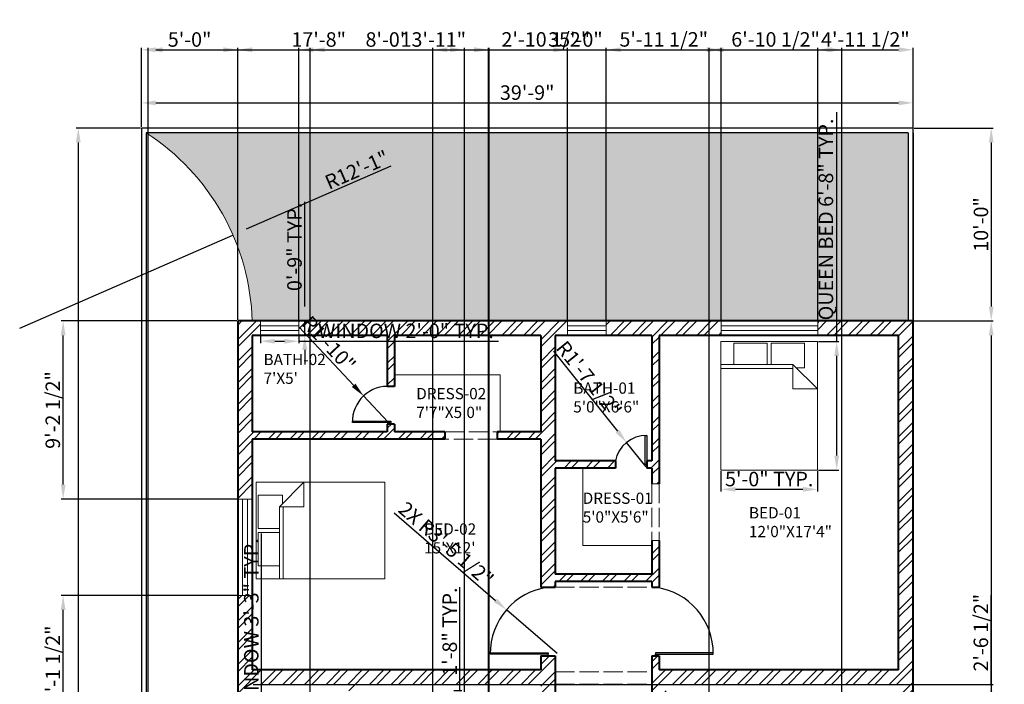
# Model space of a CAD drawing. Units: inches. Extents: x 3815 to 4442, y 1449 to 2534.
# Tile 5 of 5: x 3815 to 4428, y 2120 to 2534. Entities that reach past the tile are written whole.
import ezdxf

# ---------------------------------------------------------------- set-up
doc = ezdxf.new("R2010")
doc.units = ezdxf.units.IN
doc.linetypes.add('ACAD_ISO02W100', pattern=[15, 12, -3])
for name, color, linetype, lineweight in [('A-ANNO-DIMS', 2, 'Continuous', 18), ('A-AREA-IDEN', 7, 'Continuous', 20), ('A-DOOR', 4, 'Continuous', 25), ('A-FLOR-FIXD', 9, 'Continuous', 20), ('A-FURN', 8, 'Continuous', 18), ('A-GLAZ', 4, 'Continuous', 20), ('A-WALL', 7, 'Continuous', 40), ('A-WALL-OVHD', 8, 'ACAD_ISO02W100', 18), ('A-WALL-PATT', 8, 'Continuous', 13), ('C-PROP', 7, 'Continuous', 30), ('L-PLNT', 3, 'Continuous', 18), ('L-PLNT-PATT', 9, 'Continuous', 13)]:
    doc.layers.add(name, color=color, linetype=linetype, lineweight=lineweight)
doc.styles.get("Standard").update_dxf_attribs({"font": 'arial.ttf'})
doc.dimstyles.new('ISO-25', dxfattribs={"dimtxt": 9, "dimasz": 9, "dimexe": 1.25, "dimexo": 0.625, "dimtad": 1, "dimdec": 1, "dimrnd": 9, "dimlunit": 3, "dimtxsty": 'Standard', "dimcen": 2.5, "dimadec": 0, "dimazin": 0, "dimtfac": 1, "dimtdec": 1, "dimtmove": 0, "dimatfit": 3, "dimfxl": 1, "dimarcsym": 0})

# ---------------------------------------------------------------- blocks, each defined once
blk = doc.blocks.new('*D1')
at = {"layer": 'A-ANNO-DIMS', "color": 0, "lineweight": -2, "transparency": 16777216}
for p, q in [((3891.13, 2466.87), (3891.13, 2483.1)), ((3900.13, 2481.85), (4362.13, 2481.85)), ((4371.13, 2466.87), (4371.13, 2483.1))]:
    blk.add_line(p, q, dxfattribs=at)
at = {"layer": 'A-ANNO-DIMS', "color": 0, "lineweight": 100, "transparency": 16777216}
for points in [[(3900.13, 2483.35), (3900.13, 2480.35), (3891.13, 2481.85)], [(4362.13, 2483.35), (4362.13, 2480.35), (4371.13, 2481.85)]]:
    blk.add_solid(points, dxfattribs=at)
at = {"layer": 'Defpoints', "color": 0, "lineweight": 100, "transparency": 16777216}
for p in [(4371.13, 2481.85), (3891.13, 2466.24), (4371.13, 2466.24)]:
    blk.add_point(p, dxfattribs=at)
at = {"layer": 'A-ANNO-DIMS', "color": 0, "transparency": 16777216, "insert": (4131.13, 2487.08), "char_height": 9, "attachment_point": 5}
blk.add_mtext('39\'-9"', dxfattribs=at)
blk = doc.blocks.new('*D2')
at = {"layer": 'A-ANNO-DIMS', "color": 0, "lineweight": -2, "transparency": 16777216}
for p, q in [((3890.5, 2466.24), (3850.63, 2466.24)), ((3851.88, 2457.24), (3851.88, 1515.24)), ((3890.5, 1506.24), (3850.63, 1506.24))]:
    blk.add_line(p, q, dxfattribs=at)
at = {"layer": 'A-ANNO-DIMS', "color": 0, "lineweight": 100, "transparency": 16777216}
for points in [[(3850.38, 2457.24), (3853.38, 2457.24), (3851.88, 2466.24)], [(3850.38, 1515.24), (3853.38, 1515.24), (3851.88, 1506.24)]]:
    blk.add_solid(points, dxfattribs=at)
at = {"layer": 'Defpoints', "color": 0, "lineweight": 100, "transparency": 16777216}
for p in [(3891.13, 2466.24), (3851.88, 1506.24), (3891.13, 1506.24)]:
    blk.add_point(p, dxfattribs=at)
at = {"layer": 'A-ANNO-DIMS', "color": 0, "transparency": 16777216, "insert": (3846.65, 1986.24), "char_height": 9, "attachment_point": 5, "rotation": 90}
blk.add_mtext('80\'-3"', dxfattribs=at)
blk = doc.blocks.new('Bed - Queen')
for p, q in [((0, -80.00003), (0, 0)), ((0, 0), (59.99999, 0)), ((59.99999, 0), (59.99999, -80.00003)), ((7.99999, -1.2), (28.79998, -1.2)), ((7.99999, -14.4), (7.99999, -1.2)), ((28.79998, -1.2), (28.79998, -14.4)), ((31.19999, -1.2), (51.99999, -1.2)), ((31.19999, -14.4), (31.19999, -1.2)), ((51.99999, -1.2), (51.99999, -16.4)), ((0, -14.4), (44.8, -14.4)), ((44.8, -16.8), (0, -16.8)), ((59.99999, -29.6), (44.8, -14.4)), ((44.8, -14.4), (44.8, -29.6)), ((51.99999, -16.4), (46.79936, -16.4)), ((44.8, -29.6), (59.99999, -29.6)), ((59.99999, -80.00003), (0, -80.00003))]:
    blk.add_line(p, q)
blk = doc.blocks.new('WIN-W60-9IN')
for p, q in [((0, 9), (0, 0)), ((60, 9), (60, 0)), ((60, 6), (0, 6)), ((60, 3), (0, 3))]:
    blk.add_line(p, q)
blk = doc.blocks.new('WIN-W24-9IN')
for p, q in [((0, 9), (0, 0)), ((24, 9), (24, 0)), ((24, 6), (0, 6)), ((24, 3), (0, 3))]:
    blk.add_line(p, q)
blk = doc.blocks.new('DOOR-LEAF-24IN')
for p, q in [((0, 2), (0, 1)), ((0, 1), (24, 1)), ((0, 0), (0, 1)), ((24, 0), (0, 0)), ((24, 1), (24, 0))]:
    blk.add_line(p, q)
blk = doc.blocks.new('DOOR-LEAF-36IN')
for p, q in [((36, 2), (0, 2)), ((0, 2), (0, 1)), ((0, 0), (0, 1)), ((0, 1), (36, 1)), ((36, 1), (36, 2))]:
    blk.add_line(p, q)
blk = doc.blocks.new('*D26')
at = {"layer": 'A-ANNO-DIMS', "color": 0, "lineweight": -2, "transparency": 16777216}
for p, q in [((3965.95, 2089.9), (3965.95, 2214.04)), ((3960.75, 2089.9), (3967.2, 2089.9)), ((3965.95, 2060.05), (3965.95, 2080.9)), ((3960.75, 2051.05), (3967.2, 2051.05))]:
    blk.add_line(p, q, dxfattribs=at)
at = {"layer": 'A-ANNO-DIMS', "color": 0, "lineweight": 100, "transparency": 16777216}
for points in [[(3964.45, 2080.9), (3967.45, 2080.9), (3965.95, 2089.9)], [(3964.45, 2060.05), (3967.45, 2060.05), (3965.95, 2051.05)]]:
    blk.add_solid(points, dxfattribs=at)
at = {"layer": 'Defpoints', "color": 0, "lineweight": 100, "transparency": 16777216}
for p in [(3960.13, 2089.9), (3965.95, 2089.9), (3960.13, 2051.05)]:
    blk.add_point(p, dxfattribs=at)
at = {"layer": 'A-ANNO-DIMS', "color": 0, "transparency": 16777216, "insert": (3960.67, 2156.47), "char_height": 9, "attachment_point": 5, "rotation": 90}
blk.add_mtext('WINDOW 3\'-3" TYP.', dxfattribs=at)
blk = doc.blocks.new('*D31')
at = {"layer": 'A-ANNO-DIMS', "color": 0, "lineweight": -2, "transparency": 16777216}
for p, q in [((4089.32, 2116.41), (4089.32, 2180.67)), ((4085.45, 2116.41), (4090.57, 2116.41)), ((4089.32, 2105.41), (4089.32, 2107.41)), ((4085.45, 2096.41), (4090.57, 2096.41))]:
    blk.add_line(p, q, dxfattribs=at)
at = {"layer": 'A-ANNO-DIMS', "color": 0, "lineweight": 100, "transparency": 16777216}
for points in [[(4087.82, 2107.41), (4090.82, 2107.41), (4089.32, 2116.41)], [(4087.82, 2105.41), (4090.82, 2105.41), (4089.32, 2096.41)]]:
    blk.add_solid(points, dxfattribs=at)
at = {"layer": 'Defpoints', "color": 0, "lineweight": 100, "transparency": 16777216}
for p in [(4084.82, 2116.41), (4089.32, 2116.41), (4084.82, 2096.41)]:
    blk.add_point(p, dxfattribs=at)
at = {"layer": 'A-ANNO-DIMS', "color": 0, "transparency": 16777216, "insert": (4084.1, 2153.04), "char_height": 9, "attachment_point": 5, "rotation": 90}
blk.add_mtext('1\'-8" TYP.', dxfattribs=at)
blk = doc.blocks.new('*D32')
at = {"layer": 'A-ANNO-DIMS', "color": 0, "lineweight": -2, "transparency": 16777216}
for p, q in [((4323.66, 2333.55), (4323.66, 2476.19)), ((4312.28, 2333.55), (4324.91, 2333.55)), ((4323.66, 2262.55), (4323.66, 2324.55)), ((4312.28, 2253.55), (4324.91, 2253.55))]:
    blk.add_line(p, q, dxfattribs=at)
at = {"layer": 'A-ANNO-DIMS', "color": 0, "lineweight": 100, "transparency": 16777216}
for points in [[(4322.16, 2324.55), (4325.16, 2324.55), (4323.66, 2333.55)], [(4322.16, 2262.55), (4325.16, 2262.55), (4323.66, 2253.55)]]:
    blk.add_solid(points, dxfattribs=at)
at = {"layer": 'Defpoints', "color": 0, "lineweight": 100, "transparency": 16777216}
for p in [(4311.66, 2333.55), (4323.66, 2333.55), (4311.66, 2253.55)]:
    blk.add_point(p, dxfattribs=at)
at = {"layer": 'A-ANNO-DIMS', "color": 0, "transparency": 16777216, "insert": (4318.1, 2409.37), "char_height": 9, "attachment_point": 5, "rotation": 90}
blk.add_mtext('QUEEN BED 6\'-8" TYP.', dxfattribs=at)
blk = doc.blocks.new('*D33')
at = {"layer": 'A-ANNO-DIMS', "color": 0, "lineweight": -2, "transparency": 16777216}
for p, q in [((4251.66, 2252.92), (4251.66, 2240.3)), ((4311.66, 2252.92), (4311.66, 2240.3)), ((4260.66, 2241.55), (4302.66, 2241.55))]:
    blk.add_line(p, q, dxfattribs=at)
at = {"layer": 'A-ANNO-DIMS', "color": 0, "lineweight": 100, "transparency": 16777216}
for points in [[(4260.66, 2243.05), (4260.66, 2240.05), (4251.66, 2241.55)], [(4302.66, 2243.05), (4302.66, 2240.05), (4311.66, 2241.55)]]:
    blk.add_solid(points, dxfattribs=at)
at = {"layer": 'Defpoints', "color": 0, "lineweight": 100, "transparency": 16777216}
for p in [(4251.66, 2253.55), (4311.66, 2253.55), (4311.66, 2241.55)]:
    blk.add_point(p, dxfattribs=at)
at = {"layer": 'A-ANNO-DIMS', "color": 0, "transparency": 16777216, "insert": (4281.66, 2246.77), "char_height": 9, "attachment_point": 5}
blk.add_mtext('5\'-0" TYP.', dxfattribs=at)
blk = doc.blocks.new('*D36')
at = {"layer": 'A-ANNO-DIMS', "color": 0, "lineweight": -2, "transparency": 16777216}
for p, q in [((3965.15, 2336.62), (3965.15, 2332.39)), ((3974.15, 2333.64), (3980.15, 2333.64)), ((3989.15, 2336.62), (3989.15, 2332.39)), ((3989.15, 2333.64), (4113.29, 2333.64))]:
    blk.add_line(p, q, dxfattribs=at)
at = {"layer": 'A-ANNO-DIMS', "color": 0, "lineweight": 100, "transparency": 16777216}
for points in [[(3974.15, 2335.14), (3974.15, 2332.14), (3965.15, 2333.64)], [(3980.15, 2335.14), (3980.15, 2332.14), (3989.15, 2333.64)]]:
    blk.add_solid(points, dxfattribs=at)
at = {"layer": 'Defpoints', "color": 0, "lineweight": 100, "transparency": 16777216}
for p in [(3965.15, 2337.24), (3989.15, 2337.24), (3989.15, 2333.64)]:
    blk.add_point(p, dxfattribs=at)
at = {"layer": 'A-ANNO-DIMS', "color": 0, "transparency": 16777216, "insert": (4055.72, 2338.92), "char_height": 9, "attachment_point": 5}
blk.add_mtext('WINDOW 2\'-0" TYP.', dxfattribs=at)
blk = doc.blocks.new('*D37')
at = {"layer": 'A-ANNO-DIMS', "color": 0, "lineweight": -2, "transparency": 16777216}
for p, q in [((3992.75, 2355.24), (3992.75, 2420.35)), ((3989.77, 2346.24), (3994, 2346.24)), ((3992.75, 2337.24), (3992.75, 2346.24)), ((3989.77, 2337.24), (3994, 2337.24)), ((3992.75, 2328.24), (3992.75, 2319.24))]:
    blk.add_line(p, q, dxfattribs=at)
at = {"layer": 'A-ANNO-DIMS', "color": 0, "lineweight": 100, "transparency": 16777216}
for points in [[(3991.25, 2355.24), (3994.25, 2355.24), (3992.75, 2346.24)], [(3991.25, 2328.24), (3994.25, 2328.24), (3992.75, 2337.24)]]:
    blk.add_solid(points, dxfattribs=at)
at = {"layer": 'Defpoints', "color": 0, "lineweight": 100, "transparency": 16777216}
for p in [(3989.15, 2346.24), (3992.75, 2346.24), (3989.15, 2337.24)]:
    blk.add_point(p, dxfattribs=at)
at = {"layer": 'A-ANNO-DIMS', "color": 0, "transparency": 16777216, "insert": (3987.53, 2392.3), "char_height": 9, "attachment_point": 5, "rotation": 90}
blk.add_mtext('0\'-9" TYP.', dxfattribs=at)
blk = doc.blocks.new('*D48')
at = {"layer": 'A-ANNO-DIMS', "color": 0, "lineweight": -2, "transparency": 16777216}
for p, q in [((3891.13, 2466.87), (3891.13, 2516.14)), ((3900.13, 2514.89), (3942.13, 2514.89)), ((3951.13, 2346.87), (3951.13, 2516.14))]:
    blk.add_line(p, q, dxfattribs=at)
at = {"layer": 'A-ANNO-DIMS', "color": 0, "lineweight": 100, "transparency": 16777216}
for points in [[(3900.13, 2516.39), (3900.13, 2513.39), (3891.13, 2514.89)], [(3942.13, 2516.39), (3942.13, 2513.39), (3951.13, 2514.89)]]:
    blk.add_solid(points, dxfattribs=at)
at = {"layer": 'Defpoints', "color": 0, "lineweight": 100, "transparency": 16777216}
for p in [(3951.13, 2514.89), (3891.13, 2466.24), (3951.13, 2346.24)]:
    blk.add_point(p, dxfattribs=at)
at = {"layer": 'A-ANNO-DIMS', "color": 0, "transparency": 16777216, "insert": (3921.13, 2520.11), "char_height": 9, "attachment_point": 5}
blk.add_mtext('5\'-0"', dxfattribs=at)
blk = doc.blocks.new('*D49')
at = {"layer": 'A-ANNO-DIMS', "color": 0, "lineweight": -2, "transparency": 16777216}
for p, q in [((3951.13, 2346.87), (3951.13, 2516.14)), ((3960.13, 2514.89), (4362.13, 2514.89)), ((4371.13, 2466.87), (4371.13, 2516.14))]:
    blk.add_line(p, q, dxfattribs=at)
at = {"layer": 'A-ANNO-DIMS', "color": 0, "lineweight": 100, "transparency": 16777216}
for points in [[(3960.13, 2516.39), (3960.13, 2513.39), (3951.13, 2514.89)], [(4362.13, 2516.39), (4362.13, 2513.39), (4371.13, 2514.89)]]:
    blk.add_solid(points, dxfattribs=at)
at = {"layer": 'Defpoints', "color": 0, "lineweight": 100, "transparency": 16777216}
for p in [(4371.13, 2514.89), (4371.13, 2466.24), (3951.13, 2346.24)]:
    blk.add_point(p, dxfattribs=at)
at = {"layer": 'A-ANNO-DIMS', "color": 0, "transparency": 16777216, "insert": (4161.13, 2520.11), "char_height": 9, "attachment_point": 5}
blk.add_mtext('35\'-0"', dxfattribs=at)
blk = doc.blocks.new('*D50')
at = {"layer": 'A-ANNO-DIMS', "color": 0, "lineweight": -2, "transparency": 16777216}
for p, q in [((4371.75, 2466.24), (4421.03, 2466.24)), ((4419.78, 2457.24), (4419.78, 2355.24)), ((4371.75, 2346.24), (4421.03, 2346.24))]:
    blk.add_line(p, q, dxfattribs=at)
at = {"layer": 'A-ANNO-DIMS', "color": 0, "lineweight": 100, "transparency": 16777216}
for points in [[(4418.28, 2457.24), (4421.28, 2457.24), (4419.78, 2466.24)], [(4418.28, 2355.24), (4421.28, 2355.24), (4419.78, 2346.24)]]:
    blk.add_solid(points, dxfattribs=at)
at = {"layer": 'Defpoints', "color": 0, "lineweight": 100, "transparency": 16777216}
for p in [(4371.13, 2466.24), (4371.13, 2346.24), (4419.78, 2346.24)]:
    blk.add_point(p, dxfattribs=at)
at = {"layer": 'A-ANNO-DIMS', "color": 0, "transparency": 16777216, "insert": (4414.56, 2406.24), "char_height": 9, "attachment_point": 5, "rotation": 90}
blk.add_mtext('10\'-0"', dxfattribs=at)
blk = doc.blocks.new('*D52')
at = {"layer": 'A-ANNO-DIMS', "color": 0, "lineweight": -2, "transparency": 16777216}
for p, q in [((4371.75, 2346.24), (4421.03, 2346.24)), ((4419.78, 2337.24), (4419.78, 1643.24)), ((4371.75, 1634.24), (4421.03, 1634.24))]:
    blk.add_line(p, q, dxfattribs=at)
at = {"layer": 'A-ANNO-DIMS', "color": 0, "lineweight": 100, "transparency": 16777216}
for points in [[(4418.28, 2337.24), (4421.28, 2337.24), (4419.78, 2346.24)], [(4418.28, 1643.24), (4421.28, 1643.24), (4419.78, 1634.24)]]:
    blk.add_solid(points, dxfattribs=at)
at = {"layer": 'Defpoints', "color": 0, "lineweight": 100, "transparency": 16777216}
for p in [(4371.13, 2346.24), (4371.13, 1634.24), (4419.78, 1634.24)]:
    blk.add_point(p, dxfattribs=at)
at = {"layer": 'A-ANNO-DIMS', "color": 0, "transparency": 16777216, "insert": (4414.56, 1990.24), "char_height": 9, "attachment_point": 5, "rotation": 90}
blk.add_mtext('59\'-4"', dxfattribs=at)
blk = doc.blocks.new('*D54')
at = {"layer": 'A-ANNO-DIMS', "color": 0, "lineweight": -2, "transparency": 16777216}
for p, q in [((3996.13, 1823.37), (3996.13, 2516.14)), ((4005.13, 2514.89), (4083.13, 2514.89)), ((4092.13, 1823.37), (4092.13, 2516.14))]:
    blk.add_line(p, q, dxfattribs=at)
at = {"layer": 'A-ANNO-DIMS', "color": 0, "lineweight": 100, "transparency": 16777216}
for points in [[(4005.13, 2516.39), (4005.13, 2513.39), (3996.13, 2514.89)], [(4083.13, 2516.39), (4083.13, 2513.39), (4092.13, 2514.89)]]:
    blk.add_solid(points, dxfattribs=at)
at = {"layer": 'Defpoints', "color": 0, "lineweight": 100, "transparency": 16777216}
for p in [(4092.13, 2514.89), (3996.13, 1822.74), (4092.13, 1822.74)]:
    blk.add_point(p, dxfattribs=at)
at = {"layer": 'A-ANNO-DIMS', "color": 0, "transparency": 16777216, "insert": (4044.13, 2520.11), "char_height": 9, "attachment_point": 5}
blk.add_mtext('8\'-0"', dxfattribs=at)
blk = doc.blocks.new('*D55')
at = {"layer": 'A-ANNO-DIMS', "color": 0, "lineweight": -2, "transparency": 16777216}
for p, q in [((3950.5, 2346.24), (3841.23, 2346.24)), ((3842.48, 2244.52), (3842.48, 2337.24)), ((3950.5, 2235.52), (3841.23, 2235.52))]:
    blk.add_line(p, q, dxfattribs=at)
at = {"layer": 'A-ANNO-DIMS', "color": 0, "lineweight": 100, "transparency": 16777216}
for points in [[(3840.98, 2337.24), (3843.98, 2337.24), (3842.48, 2346.24)], [(3840.98, 2244.52), (3843.98, 2244.52), (3842.48, 2235.52)]]:
    blk.add_solid(points, dxfattribs=at)
at = {"layer": 'Defpoints', "color": 0, "lineweight": 100, "transparency": 16777216}
for p in [(3842.48, 2346.24), (3951.13, 2346.24), (3951.13, 2235.52)]:
    blk.add_point(p, dxfattribs=at)
at = {"layer": 'A-ANNO-DIMS', "color": 0, "transparency": 16777216, "insert": (3837.2, 2290.88), "char_height": 9, "attachment_point": 5, "rotation": 90}
blk.add_mtext('9\'-2 1/2"', dxfattribs=at)
blk = doc.blocks.new('*D56')
at = {"layer": 'A-ANNO-DIMS', "color": 0, "lineweight": -2, "transparency": 16777216}
for p, q in [((3950.5, 2175.52), (3841.23, 2175.52)), ((3842.48, 2098.9), (3842.48, 2166.52)), ((3950.5, 2089.9), (3841.23, 2089.9))]:
    blk.add_line(p, q, dxfattribs=at)
at = {"layer": 'A-ANNO-DIMS', "color": 0, "lineweight": 100, "transparency": 16777216}
for points in [[(3840.98, 2166.52), (3843.98, 2166.52), (3842.48, 2175.52)], [(3840.98, 2098.9), (3843.98, 2098.9), (3842.48, 2089.9)]]:
    blk.add_solid(points, dxfattribs=at)
at = {"layer": 'Defpoints', "color": 0, "lineweight": 100, "transparency": 16777216}
for p in [(3842.48, 2175.52), (3951.13, 2175.52), (3951.13, 2089.9)]:
    blk.add_point(p, dxfattribs=at)
at = {"layer": 'A-ANNO-DIMS', "color": 0, "transparency": 16777216, "insert": (3837.2, 2132.71), "char_height": 9, "attachment_point": 5, "rotation": 90}
blk.add_mtext('7\'-1 1/2"', dxfattribs=at)
blk = doc.blocks.new('*D59')
at = {"layer": 'A-ANNO-DIMS', "color": 0, "lineweight": -2, "transparency": 16777216}
for p, q in [((4311.85, 2346.87), (4311.85, 2516.14)), ((4320.85, 2514.89), (4362.13, 2514.89)), ((4371.13, 2346.87), (4371.13, 2516.14))]:
    blk.add_line(p, q, dxfattribs=at)
at = {"layer": 'A-ANNO-DIMS', "color": 0, "lineweight": 100, "transparency": 16777216}
for points in [[(4320.85, 2516.39), (4320.85, 2513.39), (4311.85, 2514.89)], [(4362.13, 2516.39), (4362.13, 2513.39), (4371.13, 2514.89)]]:
    blk.add_solid(points, dxfattribs=at)
at = {"layer": 'Defpoints', "color": 0, "lineweight": 100, "transparency": 16777216}
for p in [(4371.13, 2514.89), (4311.85, 2346.24), (4371.13, 2346.24)]:
    blk.add_point(p, dxfattribs=at)
at = {"layer": 'A-ANNO-DIMS', "color": 0, "transparency": 16777216, "insert": (4341.49, 2520.17), "char_height": 9, "attachment_point": 5}
blk.add_mtext('4\'-11 1/2"', dxfattribs=at)
blk = doc.blocks.new('*D60')
at = {"layer": 'A-ANNO-DIMS', "color": 0, "lineweight": -2, "transparency": 16777216}
for p, q in [((4180.29, 2346.87), (4180.29, 2516.14)), ((4189.29, 2514.89), (4242.85, 2514.89)), ((4251.85, 2346.87), (4251.85, 2516.14))]:
    blk.add_line(p, q, dxfattribs=at)
at = {"layer": 'A-ANNO-DIMS', "color": 0, "lineweight": 100, "transparency": 16777216}
for points in [[(4189.29, 2516.39), (4189.29, 2513.39), (4180.29, 2514.89)], [(4242.85, 2516.39), (4242.85, 2513.39), (4251.85, 2514.89)]]:
    blk.add_solid(points, dxfattribs=at)
at = {"layer": 'Defpoints', "color": 0, "lineweight": 100, "transparency": 16777216}
for p in [(4251.85, 2514.89), (4180.29, 2346.24), (4251.85, 2346.24)]:
    blk.add_point(p, dxfattribs=at)
at = {"layer": 'A-ANNO-DIMS', "color": 0, "transparency": 16777216, "insert": (4216.07, 2520.17), "char_height": 9, "attachment_point": 5}
blk.add_mtext('5\'-11 1/2"', dxfattribs=at)
blk = doc.blocks.new('*D61')
at = {"layer": 'A-ANNO-DIMS', "color": 0, "lineweight": -2, "transparency": 16777216}
for p, q in [((3989.15, 2346.87), (3989.15, 2516.14)), ((3998.15, 2514.89), (4147.29, 2514.89)), ((4156.29, 2346.87), (4156.29, 2516.14))]:
    blk.add_line(p, q, dxfattribs=at)
at = {"layer": 'A-ANNO-DIMS', "color": 0, "lineweight": 100, "transparency": 16777216}
for points in [[(3998.15, 2516.39), (3998.15, 2513.39), (3989.15, 2514.89)], [(4147.29, 2516.39), (4147.29, 2513.39), (4156.29, 2514.89)]]:
    blk.add_solid(points, dxfattribs=at)
at = {"layer": 'Defpoints', "color": 0, "lineweight": 100, "transparency": 16777216}
for p in [(4156.29, 2514.89), (3989.15, 2346.24), (4156.29, 2346.24)]:
    blk.add_point(p, dxfattribs=at)
at = {"layer": 'A-ANNO-DIMS', "color": 0, "transparency": 16777216, "insert": (4072.72, 2520.11), "char_height": 9, "attachment_point": 5}
blk.add_mtext('13\'-11"', dxfattribs=at)
blk = doc.blocks.new('*D63')
at = {"layer": 'A-ANNO-DIMS', "color": 0, "lineweight": -2, "transparency": 16777216}
for p, q in [((3895.33, 1506.87), (3895.33, 2516.14)), ((3904.33, 2514.89), (4098.56, 2514.89)), ((4107.56, 1506.87), (4107.56, 2516.14))]:
    blk.add_line(p, q, dxfattribs=at)
at = {"layer": 'A-ANNO-DIMS', "color": 0, "lineweight": 100, "transparency": 16777216}
for points in [[(3904.33, 2516.39), (3904.33, 2513.39), (3895.33, 2514.89)], [(4098.56, 2516.39), (4098.56, 2513.39), (4107.56, 2514.89)]]:
    blk.add_solid(points, dxfattribs=at)
at = {"layer": 'Defpoints', "color": 0, "lineweight": 100, "transparency": 16777216}
for p in [(4107.56, 2514.89), (3895.33, 1506.24), (4107.56, 1506.24)]:
    blk.add_point(p, dxfattribs=at)
at = {"layer": 'A-ANNO-DIMS', "color": 0, "transparency": 16777216, "insert": (4001.45, 2520.11), "char_height": 9, "attachment_point": 5}
blk.add_mtext('17\'-8"', dxfattribs=at)
blk = doc.blocks.new('*D67')
at = {"layer": 'A-ANNO-DIMS', "color": 0, "lineweight": -2, "transparency": 16777216}
for p, q in [((4419.78, 2120.24), (4419.78, 2175.54)), ((3960.75, 2120.24), (4421.03, 2120.24)), ((4419.78, 2098.9), (4419.78, 2111.24)), ((3960.75, 2089.9), (4421.03, 2089.9))]:
    blk.add_line(p, q, dxfattribs=at)
at = {"layer": 'A-ANNO-DIMS', "color": 0, "lineweight": 100, "transparency": 16777216}
for points in [[(4418.28, 2111.24), (4421.28, 2111.24), (4419.78, 2120.24)], [(4418.28, 2098.9), (4421.28, 2098.9), (4419.78, 2089.9)]]:
    blk.add_solid(points, dxfattribs=at)
at = {"layer": 'Defpoints', "color": 0, "lineweight": 100, "transparency": 16777216}
for p in [(3960.13, 2120.24), (4419.78, 2120.24), (3960.13, 2089.9)]:
    blk.add_point(p, dxfattribs=at)
at = {"layer": 'A-ANNO-DIMS', "color": 0, "transparency": 16777216, "insert": (4414.5, 2152.39), "char_height": 9, "attachment_point": 5, "rotation": 90}
blk.add_mtext('2\'-6 1/2"', dxfattribs=at)
blk = doc.blocks.new('*D73')
at = {"layer": 'A-ANNO-DIMS', "color": 0, "lineweight": -2, "transparency": 16777216}
for p, q in [((4072.48, 2029.94), (4072.48, 2516.14)), ((4081.48, 2514.89), (4098.04, 2514.89)), ((4107.04, 2029.94), (4107.04, 2516.14)), ((4107.04, 2514.89), (4169.33, 2514.89))]:
    blk.add_line(p, q, dxfattribs=at)
at = {"layer": 'A-ANNO-DIMS', "color": 0, "lineweight": 100, "transparency": 16777216}
for points in [[(4081.48, 2516.39), (4081.48, 2513.39), (4072.48, 2514.89)], [(4098.04, 2516.39), (4098.04, 2513.39), (4107.04, 2514.89)]]:
    blk.add_solid(points, dxfattribs=at)
at = {"layer": 'Defpoints', "color": 0, "lineweight": 100, "transparency": 16777216}
for p in [(4107.04, 2514.89), (4072.48, 2029.32), (4107.04, 2029.32)]:
    blk.add_point(p, dxfattribs=at)
at = {"layer": 'A-ANNO-DIMS', "color": 0, "transparency": 16777216, "insert": (4142.69, 2520.17), "char_height": 9, "attachment_point": 5}
blk.add_mtext('2\'-10 1/2"', dxfattribs=at)
blk = doc.blocks.new('*D76')
at = {"layer": 'A-ANNO-DIMS', "color": 0, "lineweight": -2, "transparency": 16777216}
for p, q in [((4244.38, 1827.87), (4244.38, 2516.14)), ((4253.38, 2514.89), (4317.89, 2514.89)), ((4326.89, 1827.87), (4326.89, 2516.14))]:
    blk.add_line(p, q, dxfattribs=at)
at = {"layer": 'A-ANNO-DIMS', "color": 0, "lineweight": 100, "transparency": 16777216}
for points in [[(4253.38, 2516.39), (4253.38, 2513.39), (4244.38, 2514.89)], [(4317.89, 2516.39), (4317.89, 2513.39), (4326.89, 2514.89)]]:
    blk.add_solid(points, dxfattribs=at)
at = {"layer": 'Defpoints', "color": 0, "lineweight": 100, "transparency": 16777216}
for p in [(4326.89, 2514.89), (4244.38, 1827.24), (4326.89, 1827.24)]:
    blk.add_point(p, dxfattribs=at)
at = {"layer": 'A-ANNO-DIMS', "color": 0, "transparency": 16777216, "insert": (4285.63, 2520.17), "char_height": 9, "attachment_point": 5}
blk.add_mtext('6\'-10 1/2"', dxfattribs=at)
blk = doc.blocks.new('*D77')
at = {"layer": 'A-ANNO-DIMS', "color": 0, "lineweight": -2, "transparency": 16777216}
for p, q in [((4046.39, 2442.56), (3956.35, 2403.25)), ((3815.44, 2341.74), (3948.11, 2399.65))]:
    blk.add_line(p, q, dxfattribs=at)
at = {"layer": 'A-ANNO-DIMS', "color": 0, "lineweight": 100, "transparency": 16777216}
blk.add_solid([(3955.75, 2404.63), (3956.96, 2401.88), (3948.11, 2399.65)], dxfattribs=at)
at = {"layer": 'Defpoints', "color": 0, "lineweight": 100, "transparency": 16777216}
for p in [(3948.11, 2399.65), (3815.44, 2341.74)]:
    blk.add_point(p, dxfattribs=at)
at = {"layer": 'A-ANNO-DIMS', "color": 0, "transparency": 16777216, "insert": (4025.65, 2439.12), "char_height": 9, "attachment_point": 5, "rotation": 23.5834}
blk.add_mtext('R12\'-1"', dxfattribs=at)
blk = doc.blocks.new('*D79')
at = {"layer": 'A-ANNO-DIMS', "color": 0, "lineweight": -2, "transparency": 16777216}
for p, q in [((4048.41, 2226.93), (4111.42, 2172.52)), ((4149.69, 2139.47), (4118.23, 2166.63))]:
    blk.add_line(p, q, dxfattribs=at)
at = {"layer": 'A-ANNO-DIMS', "color": 0, "lineweight": 100, "transparency": 16777216}
blk.add_solid([(4112.4, 2173.65), (4110.44, 2171.38), (4118.23, 2166.63)], dxfattribs=at)
at = {"layer": 'Defpoints', "color": 0, "lineweight": 100, "transparency": 16777216}
for p in [(4118.23, 2166.63), (4149.69, 2139.47)]:
    blk.add_point(p, dxfattribs=at)
at = {"layer": 'A-ANNO-DIMS', "color": 0, "transparency": 16777216, "insert": (4079.96, 2206.66), "char_height": 9, "attachment_point": 5, "rotation": 319.18966}
blk.add_mtext('2X R3\'-5 1/2"', dxfattribs=at)
blk = doc.blocks.new('*D83')
at = {"layer": 'A-ANNO-DIMS', "color": 0, "lineweight": -2, "transparency": 16777216}
for p, q in [((3989.18, 2342.55), (4023.2, 2306.21)), ((4044.43, 2283.54), (4029.35, 2299.64))]:
    blk.add_line(p, q, dxfattribs=at)
at = {"layer": 'A-ANNO-DIMS', "color": 0, "lineweight": 100, "transparency": 16777216}
blk.add_solid([(4024.3, 2307.23), (4022.11, 2305.18), (4029.35, 2299.64)], dxfattribs=at)
at = {"layer": 'Defpoints', "color": 0, "lineweight": 100, "transparency": 16777216}
for p in [(4029.35, 2299.64), (4044.43, 2283.54)]:
    blk.add_point(p, dxfattribs=at)
at = {"layer": 'A-ANNO-DIMS', "color": 0, "transparency": 16777216, "insert": (4006.92, 2331.23), "char_height": 9, "attachment_point": 5, "rotation": 313.11832}
blk.add_mtext('R1\'-10"', dxfattribs=at)
blk = doc.blocks.new('*D84')
at = {"layer": 'A-ANNO-DIMS', "color": 0, "lineweight": -2, "transparency": 16777216}
for p, q in [((4147.4, 2327.48), (4187.28, 2277.73)), ((4205.12, 2255.48), (4192.91, 2270.71))]:
    blk.add_line(p, q, dxfattribs=at)
at = {"layer": 'A-ANNO-DIMS', "color": 0, "lineweight": 100, "transparency": 16777216}
blk.add_solid([(4188.45, 2278.67), (4186.11, 2276.79), (4192.91, 2270.71)], dxfattribs=at)
at = {"layer": 'Defpoints', "color": 0, "lineweight": 100, "transparency": 16777216}
for p in [(4192.91, 2270.71), (4205.12, 2255.48)]:
    blk.add_point(p, dxfattribs=at)
at = {"layer": 'A-ANNO-DIMS', "color": 0, "transparency": 16777216, "insert": (4168.65, 2309.42), "char_height": 9, "attachment_point": 5, "rotation": 308.71642}
blk.add_mtext('R1\'-7 1/2"', dxfattribs=at)

msp = doc.modelspace()

# ---------------------------------------------------------------- hatches: boundary and pattern name
at = {"layer": 'A-WALL-PATT'}
h = msp.add_hatch(dxfattribs=at)
h.set_pattern_fill('ANSI32', color=256)
h.paths.add_polyline_path([(4156.29, 2346.24), (3989.15, 2346.24), (3989.15, 2337.24), (4044.13, 2337.24), (4044.13, 2305.59, -0.025534), (4046.38, 2305.51), (4048.63, 2305.51), (4048.63, 2337.24), (4139.63, 2337.24), (4139.63, 2277.24), (4112.45, 2277.24), (4112.45, 2272.74), (4139.63, 2272.74), (4139.63, 2180.66), (4148.63, 2180.66), (4148.63, 2184.24), (4208.63, 2184.24), (4208.63, 2180.66), (4213.13, 2180.66), (4213.13, 2209.79), (4208.63, 2209.79), (4208.63, 2188.74), (4148.63, 2188.74), (4148.63, 2254.74), (4185.97, 2254.74), (4185.97, 2259.24), (4148.63, 2259.24), (4148.63, 2337.24), (4156.29, 2337.24)])
h.paths.add_polyline_path([(4251.85, 2346.24), (4180.29, 2346.24), (4180.29, 2337.24), (4208.63, 2337.24), (4208.63, 2259.24), (4205.62, 2259.24), (4205.62, 2254.74), (4208.63, 2254.74), (4208.63, 2245.05), (4213.13, 2245.05), (4213.13, 2337.24), (4251.85, 2337.24)])
h.paths.add_polyline_path([(4371.13, 2346.24), (4311.85, 2346.24), (4311.85, 2337.24), (4362.13, 2337.24), (4362.13, 2129.24), (4213.13, 2129.24), (4213.13, 2137.97), (4208.63, 2137.97), (4208.63, 2111.87), (4217.63, 2111.87), (4217.63, 2120.24), (4362.13, 2120.24), (4362.13, 1643.24), (4318.71, 1643.24), (4318.71, 1634.24), (4371.13, 1634.24)])
h.paths.add_polyline_path([(3960.13, 2175.52), (3951.13, 2175.52), (3951.13, 2089.9), (3960.13, 2089.9), (3960.13, 2120.24), (4020.13, 2120.24), (4020.13, 2084.42), (4024.63, 2084.42), (4024.63, 2120.24), (4139.63, 2120.24), (4139.63, 2062.37), (4148.63, 2062.37), (4148.63, 2137.97), (4139.63, 2137.97), (4139.63, 2129.24), (3960.13, 2129.24)])
h.paths.add_polyline_path([(3960.13, 2272.74), (4044.13, 2272.74), (4079.8, 2272.74), (4079.8, 2277.24), (4048.63, 2277.24), (4048.63, 2282.04), (4044.13, 2282.04), (4044.13, 2277.24), (3960.13, 2277.24), (3960.13, 2337.24), (3965.15, 2337.24), (3965.15, 2346.24), (3951.13, 2346.24), (3951.13, 2235.52), (3960.13, 2235.52)])
h.paths.add_polyline_path([(4024.63, 2050.34), (4020.13, 2050.34), (4020.13, 2012.24), (3960.13, 2012.24), (3960.13, 2051.05), (3951.13, 2051.05), (3951.13, 1979.78), (3960.13, 1979.78), (3960.13, 2003.24), (4024.63, 2003.24)])
h.paths.add_polyline_path([(4217.63, 2072.24), (4208.63, 2072.24), (4208.63, 2015.24), (4362.13, 2015.24), (4362.13, 2024.24), (4217.63, 2024.24)], flags=17)
h.paths.add_polyline_path([(3960.13, 1940.92), (3951.13, 1940.92), (3951.13, 1883.13), (3960.13, 1883.13)])
h.paths.add_polyline_path([(3960.13, 1822.74), (4149.38, 1822.74), (4149.38, 1827.24), (3960.13, 1827.24), (3960.13, 1844.28), (3951.13, 1844.28), (3951.13, 1769.4), (3960.13, 1769.4)])
h.paths.add_polyline_path([(4362.13, 1827.24), (4326.89, 1827.24), (4326.89, 1818.24), (4362.13, 1818.24)], flags=17)
h.paths.add_polyline_path([(4244.38, 1827.24), (4208.63, 1827.24), (4203.18, 1827.24), (4203.18, 1822.74), (4208.63, 1822.74), (4208.63, 1812.3), (4217.63, 1812.3), (4217.63, 1818.24), (4244.38, 1818.24)])
h.paths.add_polyline_path([(4149.38, 1738.74), (4142.66, 1738.74), (4142.66, 1742.16), (4138.16, 1742.16), (4138.16, 1738.74), (4090.16, 1738.74), (4090.16, 1774.74), (4138.16, 1774.74), (4138.16, 1763.78), (4142.66, 1763.78), (4142.66, 1774.74), (4142.66, 1779.24), (4138.16, 1779.24), (4090.16, 1779.24), (4085.66, 1779.24), (4085.66, 1774.74), (4085.66, 1738.74), (3960.13, 1738.74), (3960.13, 1743.46), (3951.13, 1743.46), (3951.13, 1729.74), (4149.38, 1729.74)])
h.paths.add_polyline_path([(4136.7, 1703.49), (4136.7, 1729.74), (4127.7, 1729.74), (4127.7, 1703.49), (4127.7, 1701.02), (4181.38, 1655.79), (4183.63, 1655.79), (4208.63, 1655.79), (4208.63, 1664.79), (4183.63, 1664.79)])
h.paths.add_polyline_path([(4217.63, 1771.49), (4208.63, 1771.49), (4208.63, 1738.74), (4202.94, 1738.74), (4202.94, 1729.74), (4208.63, 1729.74), (4208.63, 1634.24), (4258.71, 1634.24), (4258.71, 1643.24), (4217.63, 1643.24)])
at = {"layer": 'L-PLNT-PATT'}
h = msp.add_hatch(dxfattribs=at)
h.set_pattern_fill('GOST_GLASS', color=256)
h.paths.add_polyline_path([(4368.13, 2463.24), (3894.13, 2463.24, -0.246049), (3960.13, 2346.24), (4368.13, 2346.24)])
h.paths.add_polyline_path([(4365.15, 1631.83), (4112.05, 1631.83), (4112.05, 1581.3), (4365.15, 1581.3)])
h.paths.add_polyline_path([(4365.15, 1581.3), (4112.05, 1581.3), (4112.05, 1511.54), (4365.15, 1511.54)])
h.paths.add_polyline_path([(4219.4, 1545.72), (4287.81, 1545.72), (4287.81, 1571.84), (4219.4, 1571.84)], flags=24)

# ---------------------------------------------------------------- linework, layer by layer
at = {"layer": 'A-DOOR'}
for p, q in [((4204.62, 2256.99), (4204.62, 2274.99)), ((4204.62, 2274.99), (4205.62, 2274.99)), ((4205.62, 2274.99), (4205.62, 2259.24)), ((4205.62, 2256.99), (4204.62, 2256.99)), ((4246.88, 2139.97), (4210.88, 2139.97)), ((4210.88, 2139.97), (4210.88, 2138.97)), ((4210.88, 2137.97), (4210.88, 2138.97)), ((4210.88, 2138.97), (4246.88, 2138.97)), ((4246.88, 2138.97), (4246.88, 2139.97))]:
    msp.add_line(p, q, dxfattribs=at)
for centre, radius, start, end in [((4044.43, 2283.54), 22.06, 84.93671, 181.29881), ((4205.12, 2255.48), 19.51, 88.53165, 168.90172), ((4149.69, 2139.47), 41.57, 97.69081, 180.68924), ((4205.31, 2139.47), 41.57, 359.31076, 82.30919)]:
    msp.add_arc(centre, radius, start, end, dxfattribs=at)
at = {"layer": 'A-FLOR-FIXD'}
for p, q in [((4048.63, 2312.65), (4114.34, 2312.65)), ((4114.34, 2312.65), (4114.34, 2277.24)), ((4165.66, 2254.74), (4165.66, 2206.67)), ((4165.66, 2206.67), (4208.63, 2206.67))]:
    msp.add_line(p, q, dxfattribs=at)
at = {"layer": 'A-WALL'}
for p, q in [((3951.13, 2346.24), (3951.13, 1729.74)), ((4371.13, 2346.24), (3951.13, 2346.24)), ((4371.13, 1634.24), (4371.13, 2346.24)), ((3960.13, 2337.24), (3960.13, 2277.24)), ((4044.13, 2337.24), (3960.13, 2337.24)), ((4044.13, 2337.24), (4044.13, 2305.51)), ((4048.63, 2337.24), (4048.63, 2305.51)), ((4139.63, 2337.24), (4048.63, 2337.24)), ((4139.63, 2337.24), (4139.63, 2277.24)), ((4148.63, 2337.24), (4148.63, 2259.24)), ((4208.63, 2337.24), (4148.63, 2337.24)), ((4208.63, 2337.24), (4208.63, 2259.24)), ((4362.13, 2337.24), (4213.13, 2337.24)), ((4213.13, 2337.24), (4213.13, 2245.05)), ((4362.13, 2129.24), (4362.13, 2337.24)), ((4048.63, 2305.51), (4044.13, 2305.51)), ((4048.63, 2282.04), (4044.13, 2282.04)), ((4044.13, 2282.04), (4044.13, 2277.24)), ((4048.63, 2282.04), (4048.63, 2277.24)), ((4044.13, 2277.24), (3960.13, 2277.24)), ((4044.13, 2272.74), (3960.13, 2272.74)), ((3960.13, 2272.74), (3960.13, 2129.24)), ((4079.8, 2272.74), (4044.13, 2272.74)), ((4079.8, 2277.24), (4048.63, 2277.24)), ((4079.8, 2277.24), (4079.8, 2272.74)), ((4139.63, 2277.24), (4112.45, 2277.24)), ((4112.45, 2277.24), (4112.45, 2272.74)), ((4139.63, 2272.74), (4112.45, 2272.74)), ((4139.63, 2272.74), (4139.63, 2180.66)), ((4185.97, 2259.24), (4148.63, 2259.24)), ((4148.63, 2254.74), (4148.63, 2188.74)), ((4185.97, 2254.74), (4148.63, 2254.74)), ((4185.97, 2259.24), (4185.97, 2254.74)), ((4208.63, 2259.24), (4205.62, 2259.24)), ((4205.62, 2259.24), (4205.62, 2254.74)), ((4208.63, 2254.74), (4205.62, 2254.74)), ((4208.63, 2254.74), (4208.63, 2245.05)), ((4208.63, 2209.79), (4208.63, 2188.74)), ((4213.13, 2209.79), (4213.13, 2180.66)), ((4208.63, 2188.74), (4148.63, 2188.74)), ((4139.63, 2180.66), (4148.63, 2180.66)), ((4208.63, 2184.24), (4148.63, 2184.24)), ((4148.63, 2184.24), (4148.63, 2180.66)), ((4208.63, 2184.24), (4208.63, 2180.66)), ((4208.63, 2180.66), (4213.13, 2180.66)), ((4139.63, 2137.97), (4148.63, 2137.97)), ((4139.63, 2137.97), (4139.63, 2129.24)), ((4148.63, 2137.97), (4148.63, 2003.24)), ((4208.63, 2137.97), (4213.13, 2137.97)), ((4208.63, 2137.97), (4208.63, 2111.87)), ((4213.13, 2137.97), (4213.13, 2129.24)), ((4139.63, 2129.24), (3960.13, 2129.24)), ((4362.13, 2129.24), (4213.13, 2129.24))]:
    msp.add_line(p, q, dxfattribs=at)
at = {"layer": 'A-WALL-OVHD'}
for p, q in [((4079.8, 2277.24), (4112.45, 2277.24)), ((4112.45, 2272.74), (4079.8, 2272.74)), ((4208.63, 2245.05), (4213.13, 2245.05)), ((4208.63, 2245.05), (4208.63, 2209.79)), ((4213.13, 2245.05), (4213.13, 2209.79)), ((4208.63, 2209.79), (4213.13, 2209.79)), ((4148.63, 2180.66), (4208.63, 2180.66)), ((4148.63, 2128.14), (4208.63, 2128.14)), ((4148.63, 2120.38), (4208.63, 2120.38))]:
    msp.add_line(p, q, dxfattribs=at)
at = {"layer": 'C-PROP'}
for p, q in [((4371.13, 2466.24), (3891.13, 2466.24)), ((3891.13, 2466.24), (3891.13, 1506.24)), ((3894.13, 2463.24), (3894.13, 1510.52)), ((4368.13, 2463.24), (3894.13, 2463.24)), ((4368.13, 2463.24), (4368.13, 2346.24)), ((4371.13, 2463.24), (4371.13, 2466.24)), ((4371.13, 2463.24), (4371.13, 2346.24))]:
    msp.add_line(p, q, dxfattribs=at)
at = {"layer": 'L-PLNT'}
msp.add_arc((3815.44, 2341.74), 144.75, 1.78148, 57.07343, dxfattribs=at)

# ---------------------------------------------------------------- block references
at = {"layer": 'A-DOOR', "rotation": 180}
msp.add_blockref('DOOR-LEAF-24IN', (4046.38, 2284.04), dxfattribs=at)
at = {"layer": 'A-DOOR', "extrusion": (0, 0, -1), "zscale": -1}
msp.add_blockref('DOOR-LEAF-36IN', (-4144.13, 2137.97), dxfattribs=at)
at = {"layer": 'A-FURN'}
msp.add_blockref('Bed - Queen', (4251.66, 2333.55), dxfattribs=at)
at = {"layer": 'A-FURN', "rotation": 90}
msp.add_blockref('Bed - Queen', (3962.59, 2185.91), dxfattribs=at)
at = {"layer": 'A-GLAZ'}
for name, p in [('WIN-W24-9IN', (3965.15, 2337.24)), ('WIN-W60-9IN', (4251.85, 2337.24))]:
    msp.add_blockref(name, p, dxfattribs=at)
for name, p, rotation in [('WIN-W24-9IN', (4180.29, 2346.24), 180), ('WIN-W60-9IN', (3960.13, 2175.52), 89.9999999999983)]:
    msp.add_blockref(name, p, dxfattribs=dict(at, rotation=rotation))

# ---------------------------------------------------------------- texts
at = {"layer": 'A-AREA-IDEN', "char_height": 7, "attachment_point": 1}
for s, insert in [("BATH-02\\P7'X5'", (3967.13, 2325.8)), ('DRESS-02\\P7\'7"X5\'0"', (4062.1, 2304.56)), ('BATH-01\\P5\'0"X6\'6"', (4159.8, 2308)), ('DRESS-01\\P5\'0"X5\'6"', (4165.66, 2239.52)), ('BED-01\\P12\'0"X17\'4"', (4269.07, 2230.46)), ("BED-02\\P15'X12'", (4067.01, 2220.36))]:
    msp.add_mtext_dynamic_manual_height_columns(s, width=62.2181, gutter_width=12.5, heights=[0], dxfattribs=dict(at, insert=insert))

# ---------------------------------------------------------------- dimensions: what is measured, and where the dimension line sits
at = {"layer": 'A-ANNO-DIMS'}
for base, p1, p2, override, picture, middle in [((4107.04, 2514.89), (4072.48, 2029.32), (4107.04, 2029.32), {"dimdec": 1, "dimlfac": 1, "dimrnd": 0, "dimzin": 1, "dimdsep": 46, "dimlunit": 4, "dimfrac": 2}, '*D73', (4142.69, 2520.17)), ((4251.85, 2514.89), (4180.29, 2346.24), (4251.85, 2346.24), {"dimdec": 1, "dimlfac": 1, "dimrnd": 0, "dimzin": 1, "dimdsep": 46, "dimlunit": 4, "dimfrac": 2}, '*D60', (4216.07, 2520.17)), ((4326.89, 2514.89), (4244.38, 1827.24), (4326.89, 1827.24), {"dimdec": 1, "dimlfac": 1, "dimrnd": 0, "dimzin": 1, "dimdsep": 46, "dimlunit": 4, "dimfrac": 2}, '*D76', (4285.63, 2520.17)), ((4371.13, 2514.89), (4311.85, 2346.24), (4371.13, 2346.24), {"dimdec": 1, "dimlfac": 1, "dimrnd": 0, "dimzin": 1, "dimdsep": 46, "dimlunit": 4, "dimfrac": 2}, '*D59', (4341.49, 2520.17)), ((3951.13, 2514.89), (3891.13, 2466.24), (3951.13, 2346.24), {"dimdec": 1, "dimlfac": 1, "dimrnd": 0, "dimzin": 1, "dimdsep": 46, "dimlunit": 4, "dimfrac": 2}, '*D48', (3921.13, 2520.11)), ((4107.56, 2514.89), (3895.33, 1506.24), (4107.56, 1506.24), {"dimdec": 1, "dimlfac": 1, "dimrnd": 0, "dimzin": 1, "dimdsep": 46, "dimlunit": 4, "dimfrac": 2}, '*D63', (4001.45, 2520.11)), ((4371.13, 2514.89), (3951.13, 2346.24), (4371.13, 2466.24), {"dimdec": 1, "dimlfac": 1, "dimrnd": 0, "dimzin": 1, "dimdsep": 46, "dimlunit": 4, "dimfrac": 2}, '*D49', (4161.13, 2520.11)), ((4156.29, 2514.89), (3989.15, 2346.24), (4156.29, 2346.24), {"dimdec": 1, "dimlfac": 1, "dimrnd": 0, "dimzin": 1, "dimdsep": 46, "dimlunit": 4, "dimfrac": 2}, '*D61', (4072.72, 2520.11)), ((4092.13, 2514.89), (3996.13, 1822.74), (4092.13, 1822.74), {"dimdec": 1, "dimlfac": 1, "dimrnd": 0, "dimzin": 1, "dimdsep": 46, "dimlunit": 4, "dimfrac": 2}, '*D54', (4044.13, 2520.11)), ((4371.13, 2481.85), (3891.13, 2466.24), (4371.13, 2466.24), {"dimclrd": 0, "dimclre": 0, "dimclrt": 0}, '*D1', (4131.13, 2487.08))]:
    dim = msp.add_linear_dim(base=base, p1=p1, p2=p2, dimstyle='ISO-25', override=override, dxfattribs=at)
    dim.commit()
    dim.dimension.update_dxf_attribs({"geometry": picture, "text_midpoint": middle})
for base, p1, p2, text, picture, middle in [((4323.66, 2333.55), (4311.66, 2253.55), (4311.66, 2333.55), 'QUEEN BED <> TYP.', '*D32', (4318.1, 2409.37)), ((3992.75, 2346.24), (3989.15, 2337.24), (3989.15, 2346.24), '<> TYP.', '*D37', (3987.53, 2392.3)), ((3965.9546, 2089.9011), (3960.1265, 2051.0475), (3960.1265, 2089.9011), 'WINDOW <> TYP.', '*D26', (3960.6699, 2156.4698)), ((4089.32, 2116.41), (4084.82, 2096.41), (4084.82, 2116.41), '<> TYP.', '*D31', (4084.1, 2153.04))]:
    dim = msp.add_linear_dim(base=base, p1=p1, p2=p2, angle=90, text=text, dimstyle='ISO-25', override={"dimdec": 1, "dimlfac": 1, "dimrnd": 0, "dimzin": 1, "dimdsep": 46, "dimlunit": 4, "dimfrac": 2}, dxfattribs=at)
    dim.commit()
    dim.dimension.update_dxf_attribs({"geometry": picture, "text_midpoint": middle})
for base, p1, p2, override, picture, middle in [((3851.88, 1506.24), (3891.13, 2466.24), (3891.13, 1506.24), {"dimclrd": 0, "dimclre": 0, "dimclrt": 0}, '*D2', (3846.65, 1986.24)), ((4419.78, 2346.24), (4371.13, 2466.24), (4371.13, 2346.24), {"dimdec": 1, "dimlfac": 1, "dimrnd": 0, "dimzin": 1, "dimdsep": 46, "dimlunit": 4, "dimfrac": 2}, '*D50', (4414.56, 2406.24)), ((3842.48, 2346.24), (3951.13, 2235.52), (3951.13, 2346.24), {"dimdec": 1, "dimlfac": 1, "dimrnd": 0, "dimzin": 1, "dimdsep": 46, "dimlunit": 4, "dimfrac": 2}, '*D55', (3837.2, 2290.88)), ((4419.78, 1634.24), (4371.13, 2346.24), (4371.13, 1634.24), {"dimdec": 1, "dimlfac": 1, "dimrnd": 0, "dimzin": 1, "dimdsep": 46, "dimlunit": 4, "dimfrac": 2}, '*D52', (4414.56, 1990.24)), ((3842.48, 2175.52), (3951.13, 2089.9), (3951.13, 2175.52), {"dimdec": 1, "dimlfac": 1, "dimrnd": 0, "dimzin": 1, "dimdsep": 46, "dimlunit": 4, "dimfrac": 2}, '*D56', (3837.2, 2132.71)), ((4419.78, 2120.24), (3960.13, 2089.9), (3960.13, 2120.24), {"dimdec": 1, "dimlfac": 1, "dimrnd": 0, "dimzin": 1, "dimdsep": 46, "dimlunit": 4, "dimfrac": 2}, '*D67', (4414.5, 2152.39))]:
    dim = msp.add_linear_dim(base=base, p1=p1, p2=p2, angle=90, dimstyle='ISO-25', override=override, dxfattribs=at)
    dim.commit()
    dim.dimension.update_dxf_attribs({"geometry": picture, "text_midpoint": middle})
dim = msp.add_radius_dim(center=(3815.44, 2341.74), mpoint=(3948.11, 2399.65), dimstyle='ISO-25', override={"dimdec": 1, "dimlfac": 1, "dimrnd": 0, "dimzin": 1, "dimdsep": 46, "dimlunit": 4, "dimfrac": 2}, dxfattribs=at)
dim.commit()
dim.dimension.update_dxf_attribs({"geometry": '*D77', "text_midpoint": (4027.7, 2434.4), "dimtype": 164})
for base, p1, p2, text, picture, middle in [((3989.15, 2333.64), (3965.15, 2337.24), (3989.15, 2337.24), 'WINDOW <> TYP.', '*D36', (4055.72, 2338.92)), ((4311.66, 2241.55), (4251.66, 2253.55), (4311.66, 2253.55), '<> TYP.', '*D33', (4281.66, 2246.77))]:
    dim = msp.add_linear_dim(base=base, p1=p1, p2=p2, text=text, dimstyle='ISO-25', override={"dimdec": 1, "dimlfac": 1, "dimrnd": 0, "dimzin": 1, "dimdsep": 46, "dimlunit": 4, "dimfrac": 2}, dxfattribs=at)
    dim.commit()
    dim.dimension.update_dxf_attribs({"geometry": picture, "text_midpoint": middle})
for center, mpoint, picture, middle in [((4044.43, 2283.54), (4029.35, 2299.64), '*D83', (4006.92, 2331.23)), ((4205.12, 2255.48), (4192.91, 2270.71), '*D84', (4168.65, 2309.42))]:
    dim = msp.add_radius_dim(center=center, mpoint=mpoint, dimstyle='ISO-25', override={"dimdec": 1, "dimlfac": 1, "dimrnd": 0, "dimzin": 1, "dimdsep": 46, "dimlunit": 4, "dimfrac": 2}, dxfattribs=at)
    dim.commit()
    dim.dimension.update_dxf_attribs({"geometry": picture, "text_midpoint": middle})
dim = msp.add_radius_dim(center=(4149.69, 2139.47), mpoint=(4118.23, 2166.63), text='2X <>', dimstyle='ISO-25', override={"dimdec": 1, "dimlfac": 1, "dimrnd": 0, "dimzin": 1, "dimdsep": 46, "dimlunit": 4, "dimfrac": 2}, dxfattribs=at)
dim.commit()
dim.dimension.update_dxf_attribs({"geometry": '*D79', "text_midpoint": (4079.96, 2206.66)})

doc.saveas('drawing.dxf')
